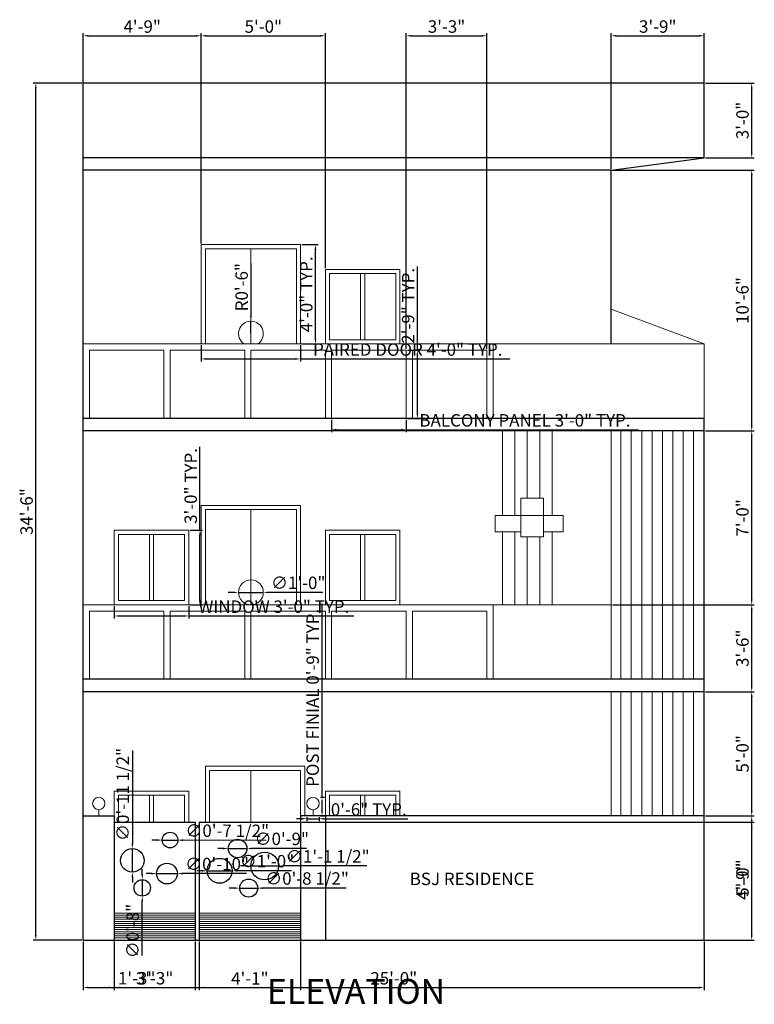
# Model space of a CAD drawing. Units: inches. Extents: x 740 to 2438, y 2555 to 3278.
# Tile 1 of 3: x 740 to 1094, y 2626 to 3102. Entities that reach past the tile are written whole.
import ezdxf

# ---------------------------------------------------------------- set-up
doc = ezdxf.new("R2010")
doc.units = ezdxf.units.IN
for name, color, linetype, lineweight in [('A-ANNO-DIMS', 2, 'Continuous', 18), ('A-ANNO-TEXT', 7, 'Continuous', 18), ('A-DOOR', 3, 'Continuous', 18), ('A-ELEV', 7, 'Continuous', 30), ('A-ELEV-DETL', 8, 'Continuous', 18), ('A-ELEV-GATE', 7, 'Continuous', 25), ('A-ELEV-PATT', 8, 'Continuous', 13), ('A-ELEV-RAIL', 7, 'Continuous', 18), ('A-GLAZ', 4, 'Continuous', 18), ('A-ROOF', 7, 'Continuous', 30)]:
    doc.layers.add(name, color=color, linetype=linetype, lineweight=lineweight)
doc.styles.get("Standard").update_dxf_attribs({"font": 'arial.ttf'})
doc.dimstyles.new('ISO-25', dxfattribs={"dimtxt": 6, "dimasz": 2.5, "dimexe": 1.25, "dimexo": 0.625, "dimtad": 1, "dimdec": 1, "dimlunit": 3, "dimtxsty": 'Standard', "dimcen": 2.5, "dimadec": 0, "dimazin": 0, "dimtfac": 1, "dimtdec": 1, "dimtmove": 0, "dimatfit": 3, "dimfxl": 1, "dimarcsym": 0})

# ---------------------------------------------------------------- blocks, each defined once
blk = doc.blocks.new('WINDOW-ELEV-36X36')
for p, q in [((17, 2), (17, 34)), ((19, 2), (19, 34))]:
    blk.add_line(p, q)
for points in [[(36, 36), (0, 36), (0, 0), (36, 0)], [(34, 34), (2, 34), (2, 2), (34, 2)]]:
    blk.add_lwpolyline(points, close=True)
blk = doc.blocks.new('DOOR-ELEV-48-PAIR')
blk.add_line((24, 46), (24, 0))
for points in [[(0, 0), (0, 48), (48, 48), (48, 0)], [(2, 0), (2, 46), (46, 46), (46, 0)]]:
    blk.add_lwpolyline(points)
blk = doc.blocks.new('POST-GLOBE')
blk.add_line((0, 0), (0, 3))
blk.add_circle((0, 6), 3)
blk = doc.blocks.new('BALCONY-PANEL-36')
for p, q in [((0, 33), (0, 0)), ((36, 33), (0, 33)), ((36, 33), (36, 0))]:
    blk.add_line(p, q)
blk = doc.blocks.new('*D14')
at = {"layer": 'A-ANNO-DIMS', "color": 0, "lineweight": -2, "transparency": 16777216}
for p, q in [((890.25, 2908.3), (890.25, 2902.28)), ((926.25, 2908.3), (926.25, 2902.28)), ((892.75, 2903.53), (923.75, 2903.53)), ((926.25, 2903.53), (1038.51, 2903.53))]:
    blk.add_line(p, q, dxfattribs=at)
at = {"layer": 'A-ANNO-DIMS', "color": 0, "transparency": 16777216}
for points in [[(892.75, 2903.94), (892.75, 2903.11), (890.25, 2903.53)], [(923.75, 2903.94), (923.75, 2903.11), (926.25, 2903.53)]]:
    blk.add_solid(points, dxfattribs=at)
at = {"layer": 'Defpoints', "color": 0, "transparency": 16777216}
for p in [(890.25, 2908.93), (926.25, 2908.93), (926.25, 2903.53)]:
    blk.add_point(p, dxfattribs=at)
at = {"layer": 'A-ANNO-DIMS', "color": 0, "transparency": 16777216, "insert": (983.63, 2907.26), "char_height": 6, "attachment_point": 5}
blk.add_mtext('BALCONY PANEL 3\'-0" TYP.', dxfattribs=at)
blk = doc.blocks.new('*D15')
at = {"layer": 'A-ANNO-DIMS', "color": 0, "lineweight": -2, "transparency": 16777216}
for p, q in [((931.65, 2941.93), (931.65, 2982.35)), ((926.88, 2941.93), (932.9, 2941.93)), ((931.65, 2911.43), (931.65, 2939.43)), ((926.88, 2908.93), (932.9, 2908.93))]:
    blk.add_line(p, q, dxfattribs=at)
at = {"layer": 'A-ANNO-DIMS', "color": 0, "transparency": 16777216}
for points in [[(931.23, 2939.43), (932.07, 2939.43), (931.65, 2941.93)], [(931.23, 2911.43), (932.07, 2911.43), (931.65, 2908.93)]]:
    blk.add_solid(points, dxfattribs=at)
at = {"layer": 'Defpoints', "color": 0, "transparency": 16777216}
for p in [(926.25, 2941.93), (931.65, 2941.93), (926.25, 2908.93)]:
    blk.add_point(p, dxfattribs=at)
at = {"layer": 'A-ANNO-DIMS', "color": 0, "transparency": 16777216, "insert": (927.96, 2963.39), "char_height": 6, "attachment_point": 5, "rotation": 90}
blk.add_mtext('2\'-9" TYP.', dxfattribs=at)
blk = doc.blocks.new('*D16')
at = {"layer": 'A-ANNO-DIMS', "color": 0, "lineweight": -2, "transparency": 16777216}
for p, q in [((785.25, 2818.3), (785.25, 2812.28)), ((821.25, 2818.3), (821.25, 2812.28)), ((787.75, 2813.53), (818.75, 2813.53)), ((821.25, 2813.53), (900.93, 2813.53))]:
    blk.add_line(p, q, dxfattribs=at)
at = {"layer": 'A-ANNO-DIMS', "color": 0, "transparency": 16777216}
for points in [[(787.75, 2813.94), (787.75, 2813.11), (785.25, 2813.53)], [(818.75, 2813.94), (818.75, 2813.11), (821.25, 2813.53)]]:
    blk.add_solid(points, dxfattribs=at)
at = {"layer": 'Defpoints', "color": 0, "transparency": 16777216}
for p in [(785.25, 2818.93), (821.25, 2818.93), (821.25, 2813.53)]:
    blk.add_point(p, dxfattribs=at)
at = {"layer": 'A-ANNO-DIMS', "color": 0, "transparency": 16777216, "insert": (862.34, 2817.26), "char_height": 6, "attachment_point": 5}
blk.add_mtext('WINDOW 3\'-0" TYP.', dxfattribs=at)
blk = doc.blocks.new('*D17')
at = {"layer": 'A-ANNO-DIMS', "color": 0, "lineweight": -2, "transparency": 16777216}
for p, q in [((826.65, 2854.93), (826.65, 2895.24)), ((821.88, 2854.93), (827.9, 2854.93)), ((826.65, 2821.43), (826.65, 2852.43)), ((821.88, 2818.93), (827.9, 2818.93))]:
    blk.add_line(p, q, dxfattribs=at)
at = {"layer": 'A-ANNO-DIMS', "color": 0, "transparency": 16777216}
for points in [[(826.23, 2852.43), (827.07, 2852.43), (826.65, 2854.93)], [(826.23, 2821.43), (827.07, 2821.43), (826.65, 2818.93)]]:
    blk.add_solid(points, dxfattribs=at)
at = {"layer": 'Defpoints', "color": 0, "transparency": 16777216}
for p in [(821.25, 2854.93), (826.65, 2854.93), (821.25, 2818.93)]:
    blk.add_point(p, dxfattribs=at)
at = {"layer": 'A-ANNO-DIMS', "color": 0, "transparency": 16777216, "insert": (822.96, 2876.33), "char_height": 6, "attachment_point": 5, "rotation": 90}
blk.add_mtext('3\'-0" TYP.', dxfattribs=at)
blk = doc.blocks.new('*D18')
at = {"layer": 'A-ANNO-DIMS', "color": 0, "lineweight": -2, "transparency": 16777216}
for p, q in [((827.25, 2944.3), (827.25, 2936.48)), ((875.25, 2944.3), (875.25, 2936.48)), ((829.75, 2937.73), (872.75, 2937.73)), ((875.25, 2937.73), (976.29, 2937.73))]:
    blk.add_line(p, q, dxfattribs=at)
at = {"layer": 'A-ANNO-DIMS', "color": 0, "transparency": 16777216}
for points in [[(829.75, 2938.14), (829.75, 2937.31), (827.25, 2937.73)], [(872.75, 2938.14), (872.75, 2937.31), (875.25, 2937.73)]]:
    blk.add_solid(points, dxfattribs=at)
at = {"layer": 'Defpoints', "color": 0, "transparency": 16777216}
for p in [(827.25, 2944.93), (875.25, 2944.93), (875.25, 2937.73)]:
    blk.add_point(p, dxfattribs=at)
at = {"layer": 'A-ANNO-DIMS', "color": 0, "transparency": 16777216, "insert": (927.02, 2941.45), "char_height": 6, "attachment_point": 5}
blk.add_mtext('PAIRED DOOR 4\'-0" TYP.', dxfattribs=at)
blk = doc.blocks.new('*D19')
at = {"layer": 'A-ANNO-DIMS', "color": 0, "lineweight": -2, "transparency": 16777216}
for p, q in [((875.88, 2992.93), (883.7, 2992.93)), ((882.45, 2947.43), (882.45, 2990.43)), ((875.88, 2944.93), (883.7, 2944.93))]:
    blk.add_line(p, q, dxfattribs=at)
at = {"layer": 'A-ANNO-DIMS', "color": 0, "transparency": 16777216}
for points in [[(882.03, 2990.43), (882.87, 2990.43), (882.45, 2992.93)], [(882.03, 2947.43), (882.87, 2947.43), (882.45, 2944.93)]]:
    blk.add_solid(points, dxfattribs=at)
at = {"layer": 'Defpoints', "color": 0, "transparency": 16777216}
for p in [(875.25, 2992.93), (882.45, 2992.93), (875.25, 2944.93)]:
    blk.add_point(p, dxfattribs=at)
at = {"layer": 'A-ANNO-DIMS', "color": 0, "transparency": 16777216, "insert": (878.76, 2968.93), "char_height": 6, "attachment_point": 5, "rotation": 90}
blk.add_mtext('4\'-0" TYP.', dxfattribs=at)
blk = doc.blocks.new('*D20')
at = {"layer": 'A-ANNO-DIMS', "color": 0, "lineweight": -2, "transparency": 16777216}
for p, q in [((885.6, 2725.93), (885.6, 2819.51)), ((884.88, 2725.93), (886.85, 2725.93)), ((885.6, 2719.43), (885.6, 2723.43)), ((884.88, 2716.93), (886.85, 2716.93))]:
    blk.add_line(p, q, dxfattribs=at)
at = {"layer": 'A-ANNO-DIMS', "color": 0, "transparency": 16777216}
for points in [[(885.18, 2723.43), (886.02, 2723.43), (885.6, 2725.93)], [(885.18, 2719.43), (886.02, 2719.43), (885.6, 2716.93)]]:
    blk.add_solid(points, dxfattribs=at)
at = {"layer": 'Defpoints', "color": 0, "transparency": 16777216}
for p in [(884.25, 2725.93), (885.6, 2725.93), (884.25, 2716.93)]:
    blk.add_point(p, dxfattribs=at)
at = {"layer": 'A-ANNO-DIMS', "color": 0, "transparency": 16777216, "insert": (881.87, 2773.97), "char_height": 6, "attachment_point": 5, "rotation": 90}
blk.add_mtext('POST FINIAL 0\'-9" TYP.', dxfattribs=at)
blk = doc.blocks.new('*D21')
at = {"layer": 'A-ANNO-DIMS', "color": 0, "lineweight": -2, "transparency": 16777216}
for p, q in [((878.25, 2716.3), (878.25, 2714.33)), ((884.25, 2716.3), (884.25, 2714.33)), ((875.75, 2715.58), (873.25, 2715.58)), ((878.25, 2715.58), (884.25, 2715.58)), ((886.75, 2715.58), (927.07, 2715.58))]:
    blk.add_line(p, q, dxfattribs=at)
at = {"layer": 'A-ANNO-DIMS', "color": 0, "transparency": 16777216}
for points in [[(875.75, 2715.99), (875.75, 2715.16), (878.25, 2715.58)], [(886.75, 2715.99), (886.75, 2715.16), (884.25, 2715.58)]]:
    blk.add_solid(points, dxfattribs=at)
at = {"layer": 'Defpoints', "color": 0, "transparency": 16777216}
for p in [(878.25, 2716.93), (884.25, 2716.93), (884.25, 2715.58)]:
    blk.add_point(p, dxfattribs=at)
at = {"layer": 'A-ANNO-DIMS', "color": 0, "transparency": 16777216, "insert": (908.16, 2719.26), "char_height": 6, "attachment_point": 5}
blk.add_mtext('0\'-6" TYP.', dxfattribs=at)
blk = doc.blocks.new('*D45')
at = {"layer": 'A-ANNO-DIMS', "color": 0, "lineweight": -2, "transparency": 16777216}
for p, q in [((770.25, 2656.3), (770.25, 2632.78)), ((1070.25, 2656.3), (1070.25, 2632.78)), ((772.75, 2634.03), (1067.75, 2634.03))]:
    blk.add_line(p, q, dxfattribs=at)
at = {"layer": 'A-ANNO-DIMS', "color": 0, "transparency": 16777216}
for points in [[(772.75, 2634.44), (772.75, 2633.61), (770.25, 2634.03)], [(1067.75, 2634.44), (1067.75, 2633.61), (1070.25, 2634.03)]]:
    blk.add_solid(points, dxfattribs=at)
at = {"layer": 'Defpoints', "color": 0, "transparency": 16777216}
for p in [(770.25, 2656.93), (1070.25, 2656.93), (1070.25, 2634.03)]:
    blk.add_point(p, dxfattribs=at)
at = {"layer": 'A-ANNO-DIMS', "color": 0, "transparency": 16777216, "insert": (920.25, 2637.71), "char_height": 6, "attachment_point": 5}
blk.add_mtext('25\'-0"', dxfattribs=at)
blk = doc.blocks.new('*D46')
at = {"layer": 'A-ANNO-DIMS', "color": 0, "lineweight": -2, "transparency": 16777216}
for p, q in [((769.63, 3070.93), (746.1, 3070.93)), ((747.35, 2659.43), (747.35, 3068.43)), ((769.63, 2656.93), (746.1, 2656.93))]:
    blk.add_line(p, q, dxfattribs=at)
at = {"layer": 'A-ANNO-DIMS', "color": 0, "transparency": 16777216}
for points in [[(746.93, 3068.43), (747.77, 3068.43), (747.35, 3070.93)], [(746.93, 2659.43), (747.77, 2659.43), (747.35, 2656.93)]]:
    blk.add_solid(points, dxfattribs=at)
at = {"layer": 'Defpoints', "color": 0, "transparency": 16777216}
for p in [(747.35, 3070.93), (770.25, 3070.93), (770.25, 2656.93)]:
    blk.add_point(p, dxfattribs=at)
at = {"layer": 'A-ANNO-DIMS', "color": 0, "transparency": 16777216, "insert": (743.66, 2863.93), "char_height": 6, "attachment_point": 5, "rotation": 90}
blk.add_mtext('34\'-6"', dxfattribs=at)
blk = doc.blocks.new('*D47')
at = {"layer": 'A-ANNO-DIMS', "color": 0, "lineweight": -2, "transparency": 16777216}
for p, q in [((1070.88, 2716.93), (1094.4, 2716.93)), ((1093.15, 2659.43), (1093.15, 2714.43)), ((1070.88, 2656.93), (1094.4, 2656.93))]:
    blk.add_line(p, q, dxfattribs=at)
at = {"layer": 'A-ANNO-DIMS', "color": 0, "transparency": 16777216}
for points in [[(1092.73, 2714.43), (1093.57, 2714.43), (1093.15, 2716.93)], [(1092.73, 2659.43), (1093.57, 2659.43), (1093.15, 2656.93)]]:
    blk.add_solid(points, dxfattribs=at)
at = {"layer": 'Defpoints', "color": 0, "transparency": 16777216}
for p in [(1070.25, 2716.93), (1093.15, 2716.93), (1070.25, 2656.93)]:
    blk.add_point(p, dxfattribs=at)
at = {"layer": 'A-ANNO-DIMS', "color": 0, "transparency": 16777216, "insert": (1089.46, 2686.93), "char_height": 6, "attachment_point": 5, "rotation": 90}
blk.add_mtext('5\'-0"', dxfattribs=at)
blk = doc.blocks.new('*D48')
at = {"layer": 'A-ANNO-DIMS', "color": 0, "lineweight": -2, "transparency": 16777216}
for p, q in [((1070.88, 2776.93), (1094.4, 2776.93)), ((1093.15, 2719.43), (1093.15, 2774.43)), ((1070.88, 2716.93), (1094.4, 2716.93))]:
    blk.add_line(p, q, dxfattribs=at)
at = {"layer": 'A-ANNO-DIMS', "color": 0, "transparency": 16777216}
for points in [[(1092.73, 2774.43), (1093.57, 2774.43), (1093.15, 2776.93)], [(1092.73, 2719.43), (1093.57, 2719.43), (1093.15, 2716.93)]]:
    blk.add_solid(points, dxfattribs=at)
at = {"layer": 'Defpoints', "color": 0, "transparency": 16777216}
for p in [(1070.25, 2776.93), (1093.15, 2776.93), (1070.25, 2716.93)]:
    blk.add_point(p, dxfattribs=at)
at = {"layer": 'A-ANNO-DIMS', "color": 0, "transparency": 16777216, "insert": (1089.46, 2746.93), "char_height": 6, "attachment_point": 5, "rotation": 90}
blk.add_mtext('5\'-0"', dxfattribs=at)
blk = doc.blocks.new('*D49')
at = {"layer": 'A-ANNO-DIMS', "color": 0, "lineweight": -2, "transparency": 16777216}
for p, q in [((1025.88, 2818.93), (1094.4, 2818.93)), ((1093.15, 2779.43), (1093.15, 2816.43)), ((1070.88, 2776.93), (1094.4, 2776.93))]:
    blk.add_line(p, q, dxfattribs=at)
at = {"layer": 'A-ANNO-DIMS', "color": 0, "transparency": 16777216}
for points in [[(1092.73, 2816.43), (1093.57, 2816.43), (1093.15, 2818.93)], [(1092.73, 2779.43), (1093.57, 2779.43), (1093.15, 2776.93)]]:
    blk.add_solid(points, dxfattribs=at)
at = {"layer": 'Defpoints', "color": 0, "transparency": 16777216}
for p in [(1025.25, 2818.93), (1093.15, 2818.93), (1070.25, 2776.93)]:
    blk.add_point(p, dxfattribs=at)
at = {"layer": 'A-ANNO-DIMS', "color": 0, "transparency": 16777216, "insert": (1089.46, 2797.93), "char_height": 6, "attachment_point": 5, "rotation": 90}
blk.add_mtext('3\'-6"', dxfattribs=at)
blk = doc.blocks.new('*D50')
at = {"layer": 'A-ANNO-DIMS', "color": 0, "lineweight": -2, "transparency": 16777216}
for p, q in [((1070.88, 2902.93), (1094.4, 2902.93)), ((1093.15, 2821.43), (1093.15, 2900.43)), ((1025.88, 2818.93), (1094.4, 2818.93))]:
    blk.add_line(p, q, dxfattribs=at)
at = {"layer": 'A-ANNO-DIMS', "color": 0, "transparency": 16777216}
for points in [[(1092.73, 2900.43), (1093.57, 2900.43), (1093.15, 2902.93)], [(1092.73, 2821.43), (1093.57, 2821.43), (1093.15, 2818.93)]]:
    blk.add_solid(points, dxfattribs=at)
at = {"layer": 'Defpoints', "color": 0, "transparency": 16777216}
for p in [(1070.25, 2902.93), (1093.15, 2902.93), (1025.25, 2818.93)]:
    blk.add_point(p, dxfattribs=at)
at = {"layer": 'A-ANNO-DIMS', "color": 0, "transparency": 16777216, "insert": (1089.46, 2860.93), "char_height": 6, "attachment_point": 5, "rotation": 90}
blk.add_mtext('7\'-0"', dxfattribs=at)
blk = doc.blocks.new('*D51')
at = {"layer": 'A-ANNO-DIMS', "color": 0, "lineweight": -2, "transparency": 16777216}
for p, q in [((1025.88, 3028.93), (1094.4, 3028.93)), ((1093.15, 2905.43), (1093.15, 3026.43)), ((1070.88, 2902.93), (1094.4, 2902.93))]:
    blk.add_line(p, q, dxfattribs=at)
at = {"layer": 'A-ANNO-DIMS', "color": 0, "transparency": 16777216}
for points in [[(1092.73, 3026.43), (1093.57, 3026.43), (1093.15, 3028.93)], [(1092.73, 2905.43), (1093.57, 2905.43), (1093.15, 2902.93)]]:
    blk.add_solid(points, dxfattribs=at)
at = {"layer": 'Defpoints', "color": 0, "transparency": 16777216}
for p in [(1025.25, 3028.93), (1093.15, 3028.93), (1070.25, 2902.93)]:
    blk.add_point(p, dxfattribs=at)
at = {"layer": 'A-ANNO-DIMS', "color": 0, "transparency": 16777216, "insert": (1089.46, 2965.93), "char_height": 6, "attachment_point": 5, "rotation": 90}
blk.add_mtext('10\'-6"', dxfattribs=at)
blk = doc.blocks.new('*D52')
at = {"layer": 'A-ANNO-DIMS', "color": 0, "lineweight": -2, "transparency": 16777216}
for p, q in [((1070.88, 3070.93), (1094.4, 3070.93)), ((1093.15, 3037.43), (1093.15, 3068.43)), ((1070.88, 3034.93), (1094.4, 3034.93))]:
    blk.add_line(p, q, dxfattribs=at)
at = {"layer": 'A-ANNO-DIMS', "color": 0, "transparency": 16777216}
for points in [[(1092.73, 3068.43), (1093.57, 3068.43), (1093.15, 3070.93)], [(1092.73, 3037.43), (1093.57, 3037.43), (1093.15, 3034.93)]]:
    blk.add_solid(points, dxfattribs=at)
at = {"layer": 'Defpoints', "color": 0, "transparency": 16777216}
for p in [(1070.25, 3070.93), (1093.15, 3070.93), (1070.25, 3034.93)]:
    blk.add_point(p, dxfattribs=at)
at = {"layer": 'A-ANNO-DIMS', "color": 0, "transparency": 16777216, "insert": (1089.46, 3052.93), "char_height": 6, "attachment_point": 5, "rotation": 90}
blk.add_mtext('3\'-0"', dxfattribs=at)
blk = doc.blocks.new('*D53')
at = {"layer": 'A-ANNO-DIMS', "color": 0, "lineweight": -2, "transparency": 16777216}
for p, q in [((1025.25, 3029.55), (1025.25, 3095.08)), ((1027.75, 3093.83), (1067.75, 3093.83)), ((1070.25, 3035.55), (1070.25, 3095.08))]:
    blk.add_line(p, q, dxfattribs=at)
at = {"layer": 'A-ANNO-DIMS', "color": 0, "transparency": 16777216}
for points in [[(1027.75, 3094.24), (1027.75, 3093.41), (1025.25, 3093.83)], [(1067.75, 3094.24), (1067.75, 3093.41), (1070.25, 3093.83)]]:
    blk.add_solid(points, dxfattribs=at)
at = {"layer": 'Defpoints', "color": 0, "transparency": 16777216}
for p in [(1070.25, 3093.83), (1070.25, 3034.93), (1025.25, 3028.93)]:
    blk.add_point(p, dxfattribs=at)
at = {"layer": 'A-ANNO-DIMS', "color": 0, "transparency": 16777216, "insert": (1047.75, 3097.52), "char_height": 6, "attachment_point": 5}
blk.add_mtext('3\'-9"', dxfattribs=at)
blk = doc.blocks.new('*D54')
at = {"layer": 'A-ANNO-DIMS', "color": 0, "lineweight": -2, "transparency": 16777216}
for p, q in [((770.25, 2656.3), (770.25, 2632.78)), ((785.25, 2656.3), (785.25, 2632.78)), ((772.75, 2634.03), (782.75, 2634.03)), ((785.25, 2634.03), (804.39, 2634.03))]:
    blk.add_line(p, q, dxfattribs=at)
at = {"layer": 'A-ANNO-DIMS', "color": 0, "transparency": 16777216}
for points in [[(772.75, 2634.44), (772.75, 2633.61), (770.25, 2634.03)], [(782.75, 2634.44), (782.75, 2633.61), (785.25, 2634.03)]]:
    blk.add_solid(points, dxfattribs=at)
at = {"layer": 'Defpoints', "color": 0, "transparency": 16777216}
for p in [(770.25, 2656.93), (785.25, 2656.93), (785.25, 2634.03)]:
    blk.add_point(p, dxfattribs=at)
at = {"layer": 'A-ANNO-DIMS', "color": 0, "transparency": 16777216, "insert": (796.07, 2637.72), "char_height": 6, "attachment_point": 5}
blk.add_mtext('1\'-3"', dxfattribs=at)
blk = doc.blocks.new('*D55')
at = {"layer": 'A-ANNO-DIMS', "color": 0, "lineweight": -2, "transparency": 16777216}
for p, q in [((770.25, 2945.55), (770.25, 3095.08)), ((772.75, 3093.83), (824.75, 3093.83)), ((827.25, 2993.55), (827.25, 3095.08))]:
    blk.add_line(p, q, dxfattribs=at)
at = {"layer": 'A-ANNO-DIMS', "color": 0, "transparency": 16777216}
for points in [[(772.75, 3094.24), (772.75, 3093.41), (770.25, 3093.83)], [(824.75, 3094.24), (824.75, 3093.41), (827.25, 3093.83)]]:
    blk.add_solid(points, dxfattribs=at)
at = {"layer": 'Defpoints', "color": 0, "transparency": 16777216}
for p in [(827.25, 3093.83), (827.25, 2992.93), (770.25, 2944.93)]:
    blk.add_point(p, dxfattribs=at)
at = {"layer": 'A-ANNO-DIMS', "color": 0, "transparency": 16777216, "insert": (798.75, 3097.51), "char_height": 6, "attachment_point": 5}
blk.add_mtext('4\'-9"', dxfattribs=at)
blk = doc.blocks.new('*D56')
at = {"layer": 'A-ANNO-DIMS', "color": 0, "lineweight": -2, "transparency": 16777216}
for p, q in [((827.25, 2993.55), (827.25, 3095.08)), ((829.75, 3093.83), (884.75, 3093.83)), ((887.25, 2981.55), (887.25, 3095.08))]:
    blk.add_line(p, q, dxfattribs=at)
at = {"layer": 'A-ANNO-DIMS', "color": 0, "transparency": 16777216}
for points in [[(829.75, 3094.24), (829.75, 3093.41), (827.25, 3093.83)], [(884.75, 3094.24), (884.75, 3093.41), (887.25, 3093.83)]]:
    blk.add_solid(points, dxfattribs=at)
at = {"layer": 'Defpoints', "color": 0, "transparency": 16777216}
for p in [(887.25, 3093.83), (827.25, 2992.93), (887.25, 2980.93)]:
    blk.add_point(p, dxfattribs=at)
at = {"layer": 'A-ANNO-DIMS', "color": 0, "transparency": 16777216, "insert": (857.25, 3097.51), "char_height": 6, "attachment_point": 5}
blk.add_mtext('5\'-0"', dxfattribs=at)
blk = doc.blocks.new('*D57')
at = {"layer": 'A-ANNO-DIMS', "color": 0, "lineweight": -2, "transparency": 16777216}
for p, q in [((926.25, 2942.55), (926.25, 3095.08)), ((928.75, 3093.83), (962.75, 3093.83)), ((965.25, 2942.55), (965.25, 3095.08))]:
    blk.add_line(p, q, dxfattribs=at)
at = {"layer": 'A-ANNO-DIMS', "color": 0, "transparency": 16777216}
for points in [[(928.75, 3094.24), (928.75, 3093.41), (926.25, 3093.83)], [(962.75, 3094.24), (962.75, 3093.41), (965.25, 3093.83)]]:
    blk.add_solid(points, dxfattribs=at)
at = {"layer": 'Defpoints', "color": 0, "transparency": 16777216}
for p in [(965.25, 3093.83), (926.25, 2941.93), (965.25, 2941.93)]:
    blk.add_point(p, dxfattribs=at)
at = {"layer": 'A-ANNO-DIMS', "color": 0, "transparency": 16777216, "insert": (945.75, 3097.52), "char_height": 6, "attachment_point": 5}
blk.add_mtext('3\'-3"', dxfattribs=at)
blk = doc.blocks.new('*D58')
at = {"layer": 'A-ANNO-DIMS', "color": 0, "lineweight": -2, "transparency": 16777216}
for p, q in [((785.25, 2656.3), (785.25, 2632.78)), ((824.25, 2656.3), (824.25, 2632.78)), ((787.75, 2634.03), (821.75, 2634.03))]:
    blk.add_line(p, q, dxfattribs=at)
at = {"layer": 'A-ANNO-DIMS', "color": 0, "transparency": 16777216}
for points in [[(787.75, 2634.44), (787.75, 2633.61), (785.25, 2634.03)], [(821.75, 2634.44), (821.75, 2633.61), (824.25, 2634.03)]]:
    blk.add_solid(points, dxfattribs=at)
at = {"layer": 'Defpoints', "color": 0, "transparency": 16777216}
for p in [(785.25, 2656.93), (824.25, 2656.93), (824.25, 2634.03)]:
    blk.add_point(p, dxfattribs=at)
at = {"layer": 'A-ANNO-DIMS', "color": 0, "transparency": 16777216, "insert": (804.75, 2637.72), "char_height": 6, "attachment_point": 5}
blk.add_mtext('3\'-3"', dxfattribs=at)
blk = doc.blocks.new('*D59')
at = {"layer": 'A-ANNO-DIMS', "color": 0, "lineweight": -2, "transparency": 16777216}
for p, q in [((826.25, 2656.3), (826.25, 2632.78)), ((875.25, 2656.3), (875.25, 2632.78)), ((828.75, 2634.03), (872.75, 2634.03))]:
    blk.add_line(p, q, dxfattribs=at)
at = {"layer": 'A-ANNO-DIMS', "color": 0, "transparency": 16777216}
for points in [[(828.75, 2634.44), (828.75, 2633.61), (826.25, 2634.03)], [(872.75, 2634.44), (872.75, 2633.61), (875.25, 2634.03)]]:
    blk.add_solid(points, dxfattribs=at)
at = {"layer": 'Defpoints', "color": 0, "transparency": 16777216}
for p in [(826.25, 2656.93), (875.25, 2656.93), (875.25, 2634.03)]:
    blk.add_point(p, dxfattribs=at)
at = {"layer": 'A-ANNO-DIMS', "color": 0, "transparency": 16777216, "insert": (850.75, 2637.66), "char_height": 6, "attachment_point": 5}
blk.add_mtext('4\'-1"', dxfattribs=at)
blk = doc.blocks.new('*D60')
at = {"layer": 'A-ANNO-DIMS', "color": 0, "lineweight": -2, "transparency": 16777216}
for p, q in [((875.88, 2713.93), (1094.4, 2713.93)), ((1093.15, 2659.43), (1093.15, 2711.43)), ((875.88, 2656.93), (1094.4, 2656.93))]:
    blk.add_line(p, q, dxfattribs=at)
at = {"layer": 'A-ANNO-DIMS', "color": 0, "transparency": 16777216}
for points in [[(1092.73, 2711.43), (1093.57, 2711.43), (1093.15, 2713.93)], [(1092.73, 2659.43), (1093.57, 2659.43), (1093.15, 2656.93)]]:
    blk.add_solid(points, dxfattribs=at)
at = {"layer": 'Defpoints', "color": 0, "transparency": 16777216}
for p in [(875.25, 2713.93), (1093.15, 2713.93), (875.25, 2656.93)]:
    blk.add_point(p, dxfattribs=at)
at = {"layer": 'A-ANNO-DIMS', "color": 0, "transparency": 16777216, "insert": (1089.46, 2685.43), "char_height": 6, "attachment_point": 5, "rotation": 90}
blk.add_mtext('4\'-9"', dxfattribs=at)
blk = doc.blocks.new('*D83')
at = {"layer": 'A-ANNO-DIMS', "color": 0, "lineweight": -2, "transparency": 16777216}
for p, q in [((848.69, 2692.76), (846.19, 2692.77)), ((851.19, 2692.76), (864.55, 2692.76)), ((907.26, 2692.76), (867.05, 2692.76))]:
    blk.add_line(p, q, dxfattribs=at)
at = {"layer": 'A-ANNO-DIMS', "color": 0, "transparency": 16777216}
for points in [[(848.69, 2693.18), (848.69, 2692.35), (851.19, 2692.76)], [(867.05, 2693.18), (867.05, 2692.35), (864.55, 2692.76)]]:
    blk.add_solid(points, dxfattribs=at)
at = {"layer": 'Defpoints', "color": 0, "transparency": 16777216}
for p in [(851.19, 2692.76), (864.55, 2692.76)]:
    blk.add_point(p, dxfattribs=at)
at = {"layer": 'A-ANNO-DIMS', "color": 0, "transparency": 16777216, "insert": (888.41, 2696.62), "char_height": 6, "attachment_point": 5, "rotation": 359.9967}
blk.add_mtext('∅1\'-1 1/2"', dxfattribs=at)
blk = doc.blocks.new('*D84')
at = {"layer": 'A-ANNO-DIMS', "color": 0, "lineweight": -2, "transparency": 16777216}
for p, q in [((827.61, 2690.42), (825.11, 2690.42)), ((830.11, 2690.42), (842.14, 2690.43)), ((870.87, 2690.43), (844.64, 2690.43))]:
    blk.add_line(p, q, dxfattribs=at)
at = {"layer": 'A-ANNO-DIMS', "color": 0, "transparency": 16777216}
for points in [[(827.61, 2690.84), (827.61, 2690.01), (830.11, 2690.42)], [(844.64, 2690.84), (844.64, 2690.01), (842.14, 2690.43)]]:
    blk.add_solid(points, dxfattribs=at)
at = {"layer": 'Defpoints', "color": 0, "transparency": 16777216}
for p in [(830.11, 2690.42), (842.14, 2690.43)]:
    blk.add_point(p, dxfattribs=at)
at = {"layer": 'A-ANNO-DIMS', "color": 0, "transparency": 16777216, "insert": (859.01, 2694.28), "char_height": 6, "attachment_point": 5, "rotation": 0.0007}
blk.add_mtext('∅1\'-0"', dxfattribs=at)
blk = doc.blocks.new('*D85')
at = {"layer": 'A-ANNO-DIMS', "color": 0, "lineweight": -2, "transparency": 16777216}
for p, q in [((842.75, 2824.93), (840.25, 2824.93)), ((845.25, 2824.93), (857.25, 2824.93)), ((885.98, 2824.92), (859.75, 2824.92))]:
    blk.add_line(p, q, dxfattribs=at)
at = {"layer": 'A-ANNO-DIMS', "color": 0, "transparency": 16777216}
for points in [[(842.75, 2825.34), (842.75, 2824.51), (845.25, 2824.93)], [(859.75, 2825.34), (859.75, 2824.51), (857.25, 2824.93)]]:
    blk.add_solid(points, dxfattribs=at)
at = {"layer": 'Defpoints', "color": 0, "transparency": 16777216}
for p in [(845.25, 2824.93), (857.25, 2824.93)]:
    blk.add_point(p, dxfattribs=at)
at = {"layer": 'A-ANNO-DIMS', "color": 0, "transparency": 16777216, "insert": (874.11, 2828.78), "char_height": 6, "attachment_point": 5, "rotation": 359.9974}
blk.add_mtext('∅1\'-0"', dxfattribs=at)
blk = doc.blocks.new('*D86')
at = {"layer": 'A-ANNO-DIMS', "color": 0, "lineweight": -2, "transparency": 16777216}
for p, q in [((793.99, 2748.49), (793.98, 2703.62)), ((793.98, 2689.75), (793.98, 2701.12)), ((793.98, 2687.25), (793.98, 2684.75))]:
    blk.add_line(p, q, dxfattribs=at)
at = {"layer": 'A-ANNO-DIMS', "color": 0, "transparency": 16777216}
for points in [[(793.57, 2703.62), (794.4, 2703.62), (793.98, 2701.12)], [(793.56, 2687.25), (794.4, 2687.25), (793.98, 2689.75)]]:
    blk.add_solid(points, dxfattribs=at)
at = {"layer": 'Defpoints', "color": 0, "transparency": 16777216}
for p in [(793.98, 2701.12), (793.98, 2689.75)]:
    blk.add_point(p, dxfattribs=at)
at = {"layer": 'A-ANNO-DIMS', "color": 0, "transparency": 16777216, "insert": (790.13, 2727.31), "char_height": 6, "attachment_point": 5, "rotation": 89.9944}
blk.add_mtext('∅0\'-11 1/2"', dxfattribs=at)
blk = doc.blocks.new('*D87')
at = {"layer": 'A-ANNO-DIMS', "color": 0, "lineweight": -2, "transparency": 16777216}
for p, q in [((803.19, 2689.09), (800.69, 2689.09)), ((805.69, 2689.09), (815.72, 2689.09)), ((849.11, 2689.09), (818.22, 2689.09))]:
    blk.add_line(p, q, dxfattribs=at)
at = {"layer": 'A-ANNO-DIMS', "color": 0, "transparency": 16777216}
for points in [[(803.19, 2689.5), (803.19, 2688.67), (805.69, 2689.09)], [(818.22, 2689.5), (818.22, 2688.67), (815.72, 2689.09)]]:
    blk.add_solid(points, dxfattribs=at)
at = {"layer": 'Defpoints', "color": 0, "transparency": 16777216}
for p in [(805.69, 2689.09), (815.72, 2689.09)]:
    blk.add_point(p, dxfattribs=at)
at = {"layer": 'A-ANNO-DIMS', "color": 0, "transparency": 16777216, "insert": (834.91, 2692.94), "char_height": 6, "attachment_point": 5, "rotation": 359.9991}
blk.add_mtext('∅0\'-10"', dxfattribs=at)
blk = doc.blocks.new('*D88')
at = {"layer": 'A-ANNO-DIMS', "color": 0, "lineweight": -2, "transparency": 16777216}
for p, q in [((837.84, 2701.2), (835.34, 2701.2)), ((840.34, 2701.2), (849.32, 2701.2)), ((878.05, 2701.2), (851.82, 2701.2))]:
    blk.add_line(p, q, dxfattribs=at)
at = {"layer": 'A-ANNO-DIMS', "color": 0, "transparency": 16777216}
for points in [[(837.84, 2701.62), (837.84, 2700.78), (840.34, 2701.2)], [(851.82, 2701.62), (851.82, 2700.78), (849.32, 2701.2)]]:
    blk.add_solid(points, dxfattribs=at)
at = {"layer": 'Defpoints', "color": 0, "transparency": 16777216}
for p in [(840.34, 2701.2), (849.32, 2701.2)]:
    blk.add_point(p, dxfattribs=at)
at = {"layer": 'A-ANNO-DIMS', "color": 0, "transparency": 16777216, "insert": (866.18, 2705.06), "char_height": 6, "attachment_point": 5, "rotation": 0.0029}
blk.add_mtext('∅0\'-9"', dxfattribs=at)
blk = doc.blocks.new('*D89')
at = {"layer": 'A-ANNO-DIMS', "color": 0, "lineweight": -2, "transparency": 16777216}
for p, q in [((843.33, 2682.07), (840.83, 2682.07)), ((845.83, 2682.07), (854.52, 2682.07)), ((897.23, 2682.07), (857.02, 2682.07))]:
    blk.add_line(p, q, dxfattribs=at)
at = {"layer": 'A-ANNO-DIMS', "color": 0, "transparency": 16777216}
for points in [[(843.33, 2682.49), (843.33, 2681.65), (845.83, 2682.07)], [(857.02, 2682.49), (857.02, 2681.65), (854.52, 2682.07)]]:
    blk.add_solid(points, dxfattribs=at)
at = {"layer": 'Defpoints', "color": 0, "transparency": 16777216}
for p in [(845.83, 2682.07), (854.52, 2682.07)]:
    blk.add_point(p, dxfattribs=at)
at = {"layer": 'A-ANNO-DIMS', "color": 0, "transparency": 16777216, "insert": (878.37, 2685.93), "char_height": 6, "attachment_point": 5, "rotation": 0.0039}
blk.add_mtext('∅0\'-8 1/2"', dxfattribs=at)
blk = doc.blocks.new('*D90')
at = {"layer": 'A-ANNO-DIMS', "color": 0, "lineweight": -2, "transparency": 16777216}
for p, q in [((798.78, 2688.65), (798.78, 2691.15)), ((798.77, 2686.15), (798.76, 2678.18)), ((798.72, 2649.46), (798.76, 2675.68))]:
    blk.add_line(p, q, dxfattribs=at)
at = {"layer": 'A-ANNO-DIMS', "color": 0, "transparency": 16777216}
for points in [[(798.36, 2688.65), (799.19, 2688.65), (798.77, 2686.15)], [(798.34, 2675.68), (799.17, 2675.68), (798.76, 2678.18)]]:
    blk.add_solid(points, dxfattribs=at)
at = {"layer": 'Defpoints', "color": 0, "transparency": 16777216}
for p in [(798.77, 2686.15), (798.76, 2678.18)]:
    blk.add_point(p, dxfattribs=at)
at = {"layer": 'A-ANNO-DIMS', "color": 0, "transparency": 16777216, "insert": (794.88, 2661.32), "char_height": 6, "attachment_point": 5, "rotation": 89.9126}
blk.add_mtext('∅0\'-8"', dxfattribs=at)
blk = doc.blocks.new('*D91')
at = {"layer": 'A-ANNO-DIMS', "color": 0, "lineweight": -2, "transparency": 16777216}
for p, q in [((805.92, 2705.26), (803.42, 2705.27)), ((808.42, 2705.26), (815.96, 2705.23)), ((858.67, 2705.08), (818.46, 2705.22))]:
    blk.add_line(p, q, dxfattribs=at)
at = {"layer": 'A-ANNO-DIMS', "color": 0, "transparency": 16777216}
for points in [[(805.92, 2705.68), (805.92, 2704.85), (808.42, 2705.26)], [(818.46, 2705.64), (818.46, 2704.8), (815.96, 2705.23)]]:
    blk.add_solid(points, dxfattribs=at)
at = {"layer": 'Defpoints', "color": 0, "transparency": 16777216}
for p in [(808.42, 2705.26), (815.96, 2705.23)]:
    blk.add_point(p, dxfattribs=at)
at = {"layer": 'A-ANNO-DIMS', "color": 0, "transparency": 16777216, "insert": (839.83, 2709.01), "char_height": 6, "attachment_point": 5, "rotation": 359.8047}
blk.add_mtext('∅0\'-7 1/2"', dxfattribs=at)
blk = doc.blocks.new('*D92')
at = {"layer": 'A-ANNO-DIMS', "color": 0, "lineweight": -2, "transparency": 16777216}
for p, q in [((851.25, 2983.87), (851.25, 2958.43)), ((851.25, 2949.93), (851.25, 2955.93))]:
    blk.add_line(p, q, dxfattribs=at)
at = {"layer": 'A-ANNO-DIMS', "color": 0, "transparency": 16777216}
blk.add_solid([(850.83, 2958.43), (851.67, 2958.43), (851.25, 2955.93)], dxfattribs=at)
at = {"layer": 'Defpoints', "color": 0, "transparency": 16777216}
for p in [(851.25, 2955.93), (851.25, 2949.93)]:
    blk.add_point(p, dxfattribs=at)
at = {"layer": 'A-ANNO-DIMS', "color": 0, "transparency": 16777216, "insert": (847.56, 2972.4), "char_height": 6, "attachment_point": 5, "rotation": 89.9974}
blk.add_mtext('R0\'-6"', dxfattribs=at)

msp = doc.modelspace()

# ---------------------------------------------------------------- hatches: boundary and pattern name
at = {"layer": 'A-ELEV-PATT'}
h = msp.add_hatch(dxfattribs=at)
h.set_pattern_fill('ANSI31', color=256, scale=1.574803, angle=45, style=0)
h.paths.add_polyline_path([(1027.75, 2782.93), (1067.75, 2782.93), (1067.75, 2902.93), (1027.75, 2902.93)])
h = msp.add_hatch(dxfattribs=at)
h.set_pattern_fill('ANSI31', color=256, scale=1.574803, angle=45, style=0)
h.paths.add_polyline_path([(1027.75, 2716.93), (1067.75, 2716.93), (1067.75, 2776.93), (1027.75, 2776.93)])
h = msp.add_hatch(dxfattribs=at)
h.set_pattern_fill('ANSI31', color=256, scale=0.3149606, angle=-45, style=0)
h.paths.add_polyline_path([(785.25, 2657.43), (824.25, 2657.43), (824.25, 2670.43), (785.25, 2670.43)])
h = msp.add_hatch(dxfattribs=at)
h.set_pattern_fill('ANSI31', color=256, scale=0.3149606, angle=-45, style=0)
h.paths.add_polyline_path([(826.25, 2657.43), (875.25, 2657.43), (875.25, 2670.43), (826.25, 2670.43)])

# ---------------------------------------------------------------- linework, layer by layer
at = {"layer": 'A-DOOR'}
msp.add_line((851.25, 2738.93), (851.25, 2713.93), dxfattribs=at)
for points in [[(829.25, 2713.93), (829.25, 2740.93), (877.25, 2740.93), (877.25, 2716.93)], [(831.25, 2713.93), (831.25, 2738.93), (875.25, 2738.93), (875.25, 2713.93)]]:
    msp.add_lwpolyline(points, dxfattribs=at)
msp.add_circle((851.25, 2824.93), 6, dxfattribs=at)
msp.add_arc((851.25, 2949.93), 6, 303.5573, 236.4427, dxfattribs=at)
at = {"layer": 'A-ELEV'}
for p, q in [((770.25, 2656.93), (770.25, 3070.93)), ((1025.25, 2944.93), (1025.25, 3028.93)), ((1070.25, 2908.93), (770.25, 2908.93)), ((875.25, 2908.93), (827.25, 2908.93)), ((1070.25, 2656.93), (1070.25, 2908.93)), ((1070.25, 2902.93), (770.25, 2902.93)), ((1070.25, 2782.93), (770.25, 2782.93)), ((1070.25, 2776.93), (770.25, 2776.93)), ((770.25, 2716.93), (785.25, 2716.93)), ((1070.25, 2716.93), (875.25, 2716.93)), ((1070.25, 2656.93), (1070.25, 2716.93)), ((770.25, 2656.93), (1070.25, 2656.93))]:
    msp.add_line(p, q, dxfattribs=at)
at = {"layer": 'A-ELEV-DETL'}
for p, q in [((972.75, 2862.01), (972.75, 2902.93)), ((978.75, 2862.01), (978.75, 2902.93)), ((984.75, 2870.49), (984.75, 2902.93)), ((990.75, 2870.49), (990.75, 2902.93)), ((996.75, 2862.01), (996.75, 2902.93)), ((1025.25, 2782.93), (1025.25, 2902.93)), ((972.75, 2818.93), (972.75, 2854.23)), ((978.75, 2818.93), (978.75, 2854.23)), ((996.75, 2818.93), (996.75, 2854.23)), ((984.75, 2818.93), (984.75, 2851.79)), ((990.75, 2818.93), (990.75, 2851.79)), ((1025.25, 2716.93), (1025.25, 2776.93))]:
    msp.add_line(p, q, dxfattribs=at)
for points in [[(981.7, 2870.49), (992.62, 2870.49), (992.62, 2862.01), (981.7, 2862.01)], [(981.7, 2862.01), (969.26, 2862.01), (969.26, 2854.23), (981.7, 2854.23)], [(992.62, 2862.01), (1002.04, 2862.01), (1002.04, 2854.23), (992.62, 2854.23)]]:
    msp.add_lwpolyline(points, close=True, dxfattribs=at)
msp.add_lwpolyline([(992.59, 2858.12), (992.59, 2851.79), (981.7, 2851.79), (981.7, 2858.12)], dxfattribs=at)
at = {"layer": 'A-ELEV-GATE'}
for p, q in [((785.25, 2716.93), (785.25, 2656.93)), ((875.25, 2716.93), (875.25, 2656.93)), ((887.25, 2716.93), (887.25, 2656.93)), ((785.25, 2713.93), (824.25, 2713.93)), ((824.25, 2713.93), (824.25, 2656.93)), ((826.25, 2713.93), (826.25, 2656.93)), ((826.25, 2713.93), (875.25, 2713.93)), ((785.25, 2656.93), (824.25, 2656.93)), ((826.25, 2656.93), (875.25, 2656.93))]:
    msp.add_line(p, q, dxfattribs=at)
for centre, radius in [((812.19, 2705.24), 3.77), ((844.83, 2701.2), 4.49), ((793.98, 2695.44), 5.69), ((857.87, 2692.76), 6.68), ((810.71, 2689.09), 5.01), ((836.13, 2690.42), 6.02), ((798.77, 2682.16), 3.98), ((850.18, 2682.07), 4.34)]:
    msp.add_circle(centre, radius, dxfattribs=at)
at = {"layer": 'A-ELEV-RAIL'}
for p, q in [((1070.25, 2944.93), (1025.25, 2961.81)), ((968.25, 2944.93), (770.25, 2944.93)), ((770.25, 2944.93), (770.25, 2908.93)), ((968.25, 2944.93), (968.25, 2908.93)), ((968.25, 2944.93), (1070.25, 2944.93)), ((1070.25, 2944.93), (1070.25, 2908.93)), ((770.25, 2818.93), (770.25, 2782.93)), ((968.25, 2818.93), (770.25, 2818.93)), ((968.25, 2815.93), (968.25, 2818.93)), ((968.25, 2818.93), (1025.25, 2818.93)), ((1070.25, 2782.93), (1070.25, 2818.93)), ((968.25, 2815.93), (968.25, 2782.93))]:
    msp.add_line(p, q, dxfattribs=at)
at = {"layer": 'A-GLAZ'}
for p, q in [((802.25, 2713.93), (802.25, 2726.93)), ((804.25, 2713.93), (804.25, 2726.93)), ((904.25, 2716.93), (904.25, 2726.93)), ((906.25, 2716.93), (906.25, 2726.93))]:
    msp.add_line(p, q, dxfattribs=at)
for points in [[(821.25, 2713.93), (821.25, 2728.93), (785.25, 2728.93), (785.25, 2692.93)], [(819.25, 2713.93), (819.25, 2726.93), (787.25, 2726.93), (787.25, 2713.93)], [(923.25, 2716.93), (923.25, 2728.93), (887.25, 2728.93), (887.25, 2716.93)], [(921.25, 2716.93), (921.25, 2726.93), (889.25, 2726.93), (889.25, 2716.93)]]:
    msp.add_lwpolyline(points, dxfattribs=at)
at = {"layer": 'A-ROOF'}
for p, q in [((1070.25, 3070.93), (770.25, 3070.93)), ((1070.25, 3034.93), (1070.25, 3070.93)), ((1070.25, 3034.93), (770.25, 3034.93)), ((1025.25, 3028.93), (1070.25, 3034.93)), ((1025.25, 3028.93), (770.25, 3028.93))]:
    msp.add_line(p, q, dxfattribs=at)

# ---------------------------------------------------------------- block references
at = {"layer": 'A-DOOR'}
for p in [(827.25, 2944.93), (827.25, 2818.93)]:
    msp.add_blockref('DOOR-ELEV-48-PAIR', p, dxfattribs=at)
at = {"layer": 'A-ELEV-DETL'}
for p in [(777.75, 2716.93), (881.25, 2716.93)]:
    msp.add_blockref('POST-GLOBE', p, dxfattribs=at)
at = {"layer": 'A-ELEV-RAIL'}
for p in [(773.25, 2908.93), (812.25, 2908.93), (851.25, 2908.93), (890.25, 2908.93), (929.25, 2908.93), (773.25, 2782.93), (812.25, 2782.93), (851.25, 2782.93), (890.25, 2782.93), (929.25, 2782.93)]:
    msp.add_blockref('BALCONY-PANEL-36', p, dxfattribs=at)
at = {"layer": 'A-GLAZ'}
for p in [(887.25, 2944.93), (785.25, 2818.93), (887.25, 2818.93)]:
    msp.add_blockref('WINDOW-ELEV-36X36', p, dxfattribs=at)

# ---------------------------------------------------------------- texts
at = {"layer": 'A-ANNO-TEXT'}
for s, height, p in [('BSJ RESIDENCE', 6, (927.98, 2683.52)), ('ELEVATION', 12, (858.98, 2626.14))]:
    msp.add_text(s, height=height, dxfattribs=at).set_placement(p)

# ---------------------------------------------------------------- dimensions: what is measured, and where the dimension line sits
at = {"layer": 'A-ANNO-DIMS'}
for base, p1, p2, picture, middle in [((827.25, 3093.83), (770.25, 2944.93), (827.25, 2992.93), '*D55', (798.75, 3097.51)), ((887.25, 3093.83), (827.25, 2992.93), (887.25, 2980.93), '*D56', (857.25, 3097.51)), ((965.25, 3093.83), (926.25, 2941.93), (965.25, 2941.93), '*D57', (945.75, 3097.52)), ((1070.25, 3093.83), (1025.25, 3028.93), (1070.25, 3034.93), '*D53', (1047.75, 3097.52)), ((1070.25, 2634.03), (770.25, 2656.93), (1070.25, 2656.93), '*D45', (920.25, 2637.71)), ((785.25, 2634.03), (770.25, 2656.93), (785.25, 2656.93), '*D54', (796.07, 2637.72)), ((824.25, 2634.03), (785.25, 2656.93), (824.25, 2656.93), '*D58', (804.75, 2637.72)), ((875.25, 2634.03), (826.25, 2656.93), (875.25, 2656.93), '*D59', (850.75, 2637.66))]:
    dim = msp.add_linear_dim(base=base, p1=p1, p2=p2, dimstyle='ISO-25', override={"dimdec": 1, "dimlfac": 1, "dimrnd": 0, "dimzin": 1, "dimdsep": 46, "dimlunit": 4, "dimfrac": 2}, dxfattribs=at)
    dim.commit()
    dim.dimension.update_dxf_attribs({"geometry": picture, "text_midpoint": middle})
for base, p1, p2, picture, middle in [((747.35, 3070.93), (770.25, 2656.93), (770.25, 3070.93), '*D46', (743.66, 2863.93)), ((1093.15, 3070.93), (1070.25, 3034.93), (1070.25, 3070.93), '*D52', (1089.46, 3052.93)), ((1093.15, 3028.93), (1070.25, 2902.93), (1025.25, 3028.93), '*D51', (1089.46, 2965.93)), ((1093.15, 2902.93), (1025.25, 2818.93), (1070.25, 2902.93), '*D50', (1089.46, 2860.93)), ((1093.15, 2818.93), (1070.25, 2776.93), (1025.25, 2818.93), '*D49', (1089.46, 2797.93)), ((1093.15, 2776.93), (1070.25, 2716.93), (1070.25, 2776.93), '*D48', (1089.46, 2746.93)), ((1093.15, 2716.93), (1070.25, 2656.93), (1070.25, 2716.93), '*D47', (1089.46, 2686.93)), ((1093.15, 2713.93), (875.25, 2656.93), (875.25, 2713.93), '*D60', (1089.46, 2685.43))]:
    dim = msp.add_linear_dim(base=base, p1=p1, p2=p2, angle=90, dimstyle='ISO-25', override={"dimdec": 1, "dimlfac": 1, "dimrnd": 0, "dimzin": 1, "dimdsep": 46, "dimlunit": 4, "dimfrac": 2}, dxfattribs=at)
    dim.commit()
    dim.dimension.update_dxf_attribs({"geometry": picture, "text_midpoint": middle})
for base, p1, p2, text, picture, middle in [((882.45, 2992.93), (875.25, 2944.93), (875.25, 2992.93), '<> TYP.', '*D19', (878.76, 2968.93)), ((931.65, 2941.93), (926.25, 2908.93), (926.25, 2941.93), '<> TYP.', '*D15', (927.96, 2963.39)), ((826.65, 2854.93), (821.25, 2818.93), (821.25, 2854.93), '<> TYP.', '*D17', (822.96, 2876.33)), ((885.6, 2725.93), (884.25, 2716.93), (884.25, 2725.93), 'POST FINIAL <> TYP.', '*D20', (881.87, 2773.97))]:
    dim = msp.add_linear_dim(base=base, p1=p1, p2=p2, angle=90, text=text, dimstyle='ISO-25', override={"dimdec": 1, "dimlfac": 1, "dimrnd": 0, "dimzin": 1, "dimdsep": 46, "dimlunit": 4, "dimfrac": 2}, dxfattribs=at)
    dim.commit()
    dim.dimension.update_dxf_attribs({"geometry": picture, "text_midpoint": middle})
dim = msp.add_radius_dim(center=(851.25, 2949.93), mpoint=(851.25, 2955.93), dimstyle='ISO-25', override={"dimdec": 1, "dimlfac": 1, "dimrnd": 0, "dimzin": 1, "dimdsep": 46, "dimlunit": 4, "dimfrac": 2}, dxfattribs=at)
dim.commit()
dim.dimension.update_dxf_attribs({"geometry": '*D92', "text_midpoint": (847.56, 2972.4)})
for base, p1, p2, text, picture, middle in [((875.25, 2937.73), (827.25, 2944.93), (875.25, 2944.93), 'PAIRED DOOR <> TYP.', '*D18', (927.02, 2941.45)), ((926.25, 2903.53), (890.25, 2908.93), (926.25, 2908.93), 'BALCONY PANEL <> TYP.', '*D14', (983.63, 2907.26)), ((821.25, 2813.53), (785.25, 2818.93), (821.25, 2818.93), 'WINDOW <> TYP.', '*D16', (862.34, 2817.26)), ((884.25, 2715.58), (878.25, 2716.93), (884.25, 2716.93), '<> TYP.', '*D21', (908.16, 2719.26))]:
    dim = msp.add_linear_dim(base=base, p1=p1, p2=p2, text=text, dimstyle='ISO-25', override={"dimdec": 1, "dimlfac": 1, "dimrnd": 0, "dimzin": 1, "dimdsep": 46, "dimlunit": 4, "dimfrac": 2}, dxfattribs=at)
    dim.commit()
    dim.dimension.update_dxf_attribs({"geometry": picture, "text_midpoint": middle})
for p1, p2, picture, middle in [((845.25, 2824.93), (857.25, 2824.93), '*D85', (874.11, 2824.92)), ((851.19, 2692.76), (864.55, 2692.76), '*D83', (888.41, 2692.76)), ((830.11, 2690.42), (842.14, 2690.42), '*D84', (859.01, 2690.43)), ((845.83, 2682.07), (854.52, 2682.07), '*D89', (878.38, 2682.07)), ((798.77, 2686.15), (798.76, 2678.18), '*D90', (798.73, 2661.32))]:
    dim = msp.add_diameter_dim_2p(p1=p1, p2=p2, dimstyle='ISO-25', override={"dimdec": 1, "dimlfac": 1, "dimrnd": 0, "dimzin": 1, "dimdsep": 46, "dimlunit": 4, "dimfrac": 2}, dxfattribs=at)
    dim.commit()
    dim.dimension.update_dxf_attribs({"geometry": picture, "text_midpoint": middle})
for p1, p2, picture, middle in [((793.98, 2689.75), (793.98, 2701.12), '*D86', (793.99, 2727.31)), ((808.42, 2705.26), (815.96, 2705.23), '*D91', (839.82, 2705.15)), ((840.34, 2701.2), (849.32, 2701.2), '*D88', (866.18, 2701.2)), ((805.69, 2689.09), (815.72, 2689.09), '*D87', (834.91, 2689.09))]:
    dim = msp.add_diameter_dim_2p(p1=p1, p2=p2, dimstyle='ISO-25', override={"dimdec": 1, "dimlfac": 1, "dimrnd": 0, "dimzin": 1, "dimdsep": 46, "dimlunit": 4, "dimfrac": 2}, dxfattribs=at)
    dim.commit()
    dim.dimension.update_dxf_attribs({"geometry": picture, "text_midpoint": middle, "dimtype": 163})

doc.saveas('drawing.dxf')
